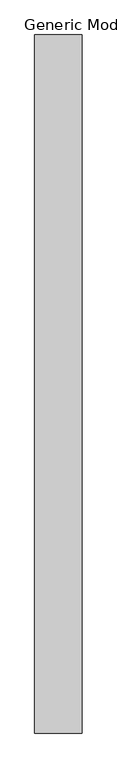
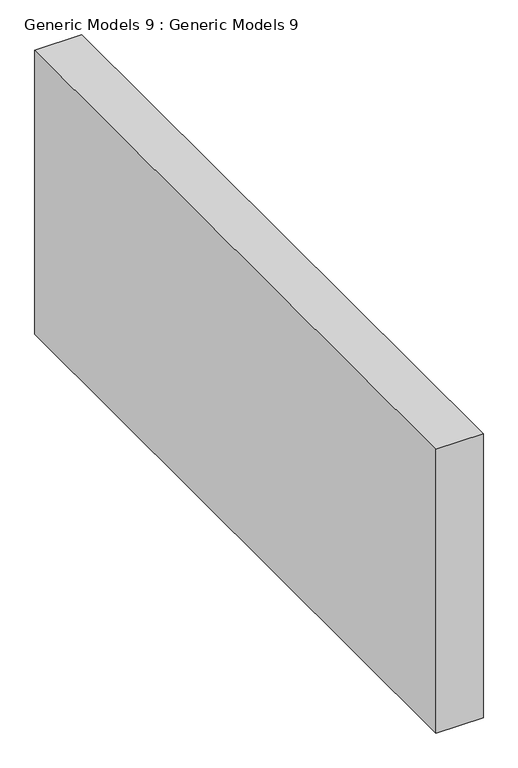
"""IFC4 building model written with IfcOpenShell, lengths in millimetres: proxy geometry, Generic Models 9 : Generic Models 9."""

from ifc_helpers import new_model, si_unit, frame, origin, place, context, project, spatial, polyline, outline, extrude, source, transform, mapped, element, save


def generic_models_9_generic_models_9_b27368f7(model_context):
    return source(origin(), model_context, "Body", "SweptSolid", [
        extrude(outline(polyline([(-4696.3466301, 5909.0031952), (-4696.3466301, 4030.8322722), (-4823.3466301, 4030.8322722), (-4823.3466301, 5909.0031952), (-4696.3466301, 5909.0031952)])), frame((0.0, 0.0, 3555.713428), z_axis=(0.0, 0.0, 1.0), x_axis=(1.0, 0.0, 0.0)), (0.0, 0.0, 1.0), 809.8357384),
    ])


if __name__ == "__main__":
    model = new_model("IFC4")
    model_context = context("Model", 3, world=origin())
    ifc_project = project(units=[si_unit("LENGTHUNIT", "METRE", prefix="MILLI")], contexts=[model_context])
    site = spatial("IfcSite", under=ifc_project)
    building = spatial("IfcBuilding", under=site)
    placement = place(None, origin())
    generic_models_9_generic_models_9_shape = generic_models_9_generic_models_9_b27368f7(model_context)
    element("IfcBuildingElementProxy", 1, Name="Generic Models 9 : Generic Models 9", ObjectType="Generic Models 9 : Generic Models 9", at=placement, inside=building, context=model_context, shape_type="MappedRepresentation", body=[
        mapped(generic_models_9_generic_models_9_shape, transform((0.0, 0.0, 0.0), x_axis=(1.0, 0.0, 0.0), y_axis=(0.0, 1.0, 0.0), z_axis=(0.0, 0.0, 1.0))),
    ])
    save(model, "model.ifc")
